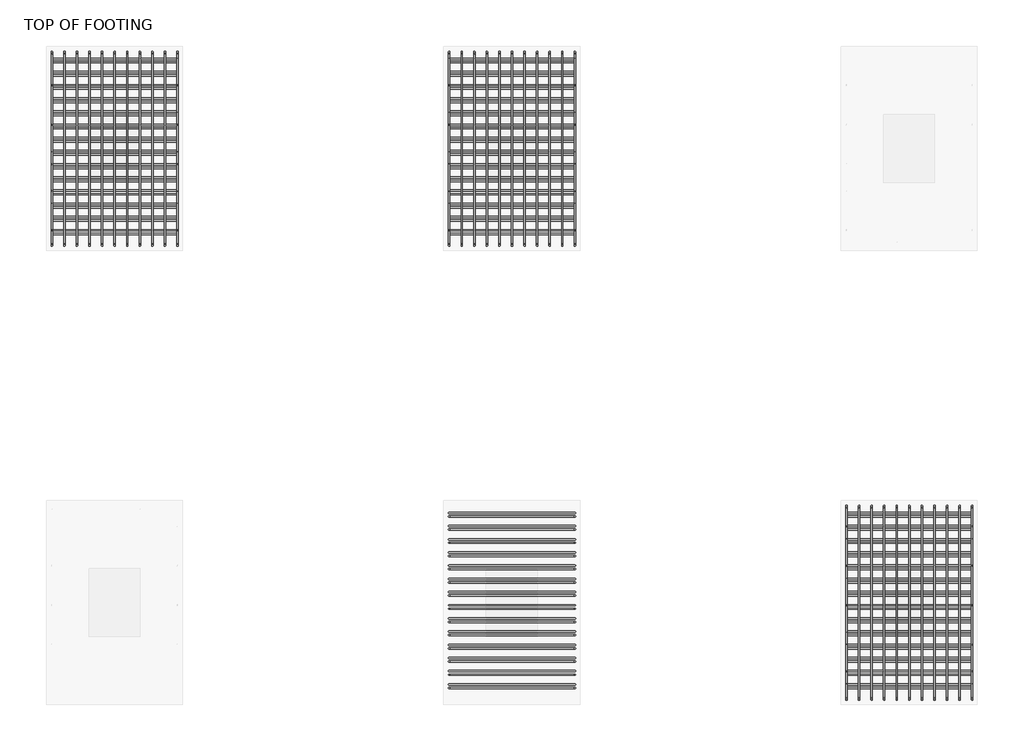
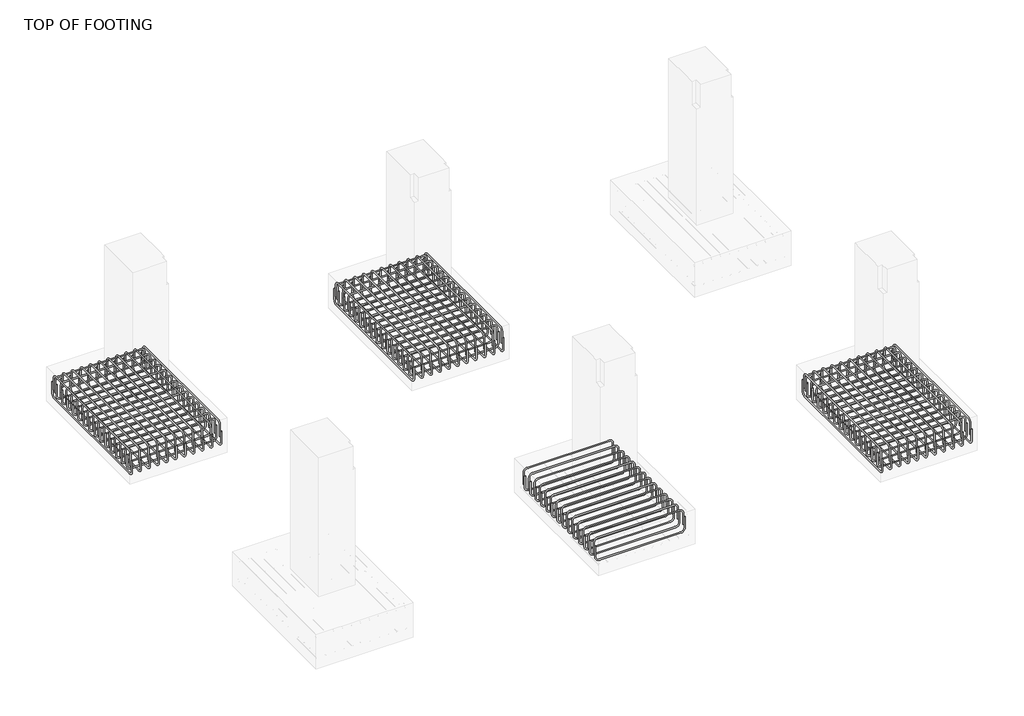
# One storey, part 6 of 11: 14 reinforcing bars.
"""IFC4 building model written with IfcOpenShell, lengths in millimetres."""

from ifc_helpers import new_model, si_unit, point, frame, origin, place, context, project, spatial, polyline, circle_curve, trimmed, segment, composite_curve, source, transform, mapped, element, save
from ifc_brep_helpers import swept_disk

model = new_model("IFC4")

# Units and contexts
model_context = context("Model", 3, world=origin())
ifc_project = project(units=[si_unit("LENGTHUNIT", "METRE", prefix="MILLI")], contexts=[model_context])

# Site, building, storey
site = spatial("IfcSite", under=ifc_project)
building = spatial("IfcBuilding", under=site)
storey = spatial("IfcBuildingStorey", under=building, Name="TOP OF FOOTING", Elevation=-1828.8)

# Reinforcing bars
placement = place(None, origin())
reinforcing_bar_shape = source(origin(), model_context, "Body", "SolidModel", [
    swept_disk(composite_curve([segment(polyline([(-8816.2384094, 18549.4712443, -2012.1658531), (-8816.2384094, 18549.4712443, -2159.4658531)]), True, "CONTINUOUS"), segment(trimmed(circle_curve(frame((-8816.2384094, 18595.8212443, -2159.4658531), z_axis=(1.0, 0.0, 0.0), x_axis=(0.0, -46.35000000000218, 0.0)), 46.35), [point((-8816.2384094, 18549.4712443, -2159.4658531))], [point((-8816.2384094, 18595.8212443, -2205.8158531))], True, "CARTESIAN"), True, "CONTINUOUS"), segment(polyline([(-8816.2384094, 18595.8212443, -2205.8158531), (-8816.2384094, 20210.4212443, -2205.8158531)]), True, "CONTINUOUS"), segment(trimmed(circle_curve(frame((-8816.2384094, 20210.4212443, -2159.4658531), z_axis=(1.0, 0.0, 0.0), x_axis=(0.0, 0.0, -46.34999999999991)), 46.35), [point((-8816.2384094, 20210.4212443, -2205.8158531))], [point((-8816.2384094, 20256.7712443, -2159.4658531))], True, "CARTESIAN"), True, "CONTINUOUS"), segment(polyline([(-8816.2384094, 20256.7712443, -2159.4658531), (-8816.2384094, 20256.7712443, -2012.1658531)]), True, "CONTINUOUS")], self_intersect=False), 6.35),
])
element("IfcReinforcingBar", 1, at=placement, inside=storey, context=model_context, shape_type="MappedRepresentation", body=[
    mapped(reinforcing_bar_shape, transform((0.0, 0.0, 0.0), x_axis=(1.0, 0.0, 0.0), y_axis=(0.0, 1.0, 0.0), z_axis=(0.0, 0.0, 1.0))),
    mapped(reinforcing_bar_shape, transform((-110.73, 0.0, 0.0), x_axis=(1.0, 0.0, 0.0), y_axis=(0.0, 1.0, 0.0), z_axis=(0.0, 0.0, 1.0))),
    mapped(reinforcing_bar_shape, transform((-221.46, 0.0, 0.0), x_axis=(1.0, 0.0, 0.0), y_axis=(0.0, 1.0, 0.0), z_axis=(0.0, 0.0, 1.0))),
    mapped(reinforcing_bar_shape, transform((-332.19, 0.0, 0.0), x_axis=(1.0, 0.0, 0.0), y_axis=(0.0, 1.0, 0.0), z_axis=(0.0, 0.0, 1.0))),
    mapped(reinforcing_bar_shape, transform((-442.92, 0.0, 0.0), x_axis=(1.0, 0.0, 0.0), y_axis=(0.0, 1.0, 0.0), z_axis=(0.0, 0.0, 1.0))),
    mapped(reinforcing_bar_shape, transform((-553.65, 0.0, 0.0), x_axis=(1.0, 0.0, 0.0), y_axis=(0.0, 1.0, 0.0), z_axis=(0.0, 0.0, 1.0))),
    mapped(reinforcing_bar_shape, transform((-664.38, 0.0, 0.0), x_axis=(1.0, 0.0, 0.0), y_axis=(0.0, 1.0, 0.0), z_axis=(0.0, 0.0, 1.0))),
    mapped(reinforcing_bar_shape, transform((-775.11, 0.0, 0.0), x_axis=(1.0, 0.0, 0.0), y_axis=(0.0, 1.0, 0.0), z_axis=(0.0, 0.0, 1.0))),
    mapped(reinforcing_bar_shape, transform((-885.84, 0.0, 0.0), x_axis=(1.0, 0.0, 0.0), y_axis=(0.0, 1.0, 0.0), z_axis=(0.0, 0.0, 1.0))),
    mapped(reinforcing_bar_shape, transform((-996.57, 0.0, 0.0), x_axis=(1.0, 0.0, 0.0), y_axis=(0.0, 1.0, 0.0), z_axis=(0.0, 0.0, 1.0))),
    mapped(reinforcing_bar_shape, transform((-1107.3, 0.0, 0.0), x_axis=(1.0, 0.0, 0.0), y_axis=(0.0, 1.0, 0.0), z_axis=(0.0, 0.0, 1.0))),
])
reinforcing_bar_2_shape = source(origin(), model_context, "Body", "SolidModel", [
    swept_disk(composite_curve([segment(polyline([(-9923.5384094, 18577.6603603, -2096.8914539), (-9923.5384094, 18577.6603603, -1949.5914539)]), True, "CONTINUOUS"), segment(trimmed(circle_curve(frame((-9923.5384094, 18624.0103603, -1949.5914539), z_axis=(-1.0, 0.0, 0.0), x_axis=(0.0, -46.349999999998545, 0.0)), 46.35), [point((-9923.5384094, 18577.6603603, -1949.5914539))], [point((-9923.5384094, 18624.0103603, -1903.2414539))], True, "CARTESIAN"), True, "CONTINUOUS"), segment(polyline([(-9923.5384094, 18624.0103603, -1903.2414539), (-9923.5384094, 20181.3238837, -1903.2414539)]), True, "CONTINUOUS"), segment(trimmed(circle_curve(frame((-9923.5384094, 20181.3238837, -1949.5914539), z_axis=(-1.0, 0.0, 0.0), x_axis=(0.0, 0.0, 46.350000000000136)), 46.35), [point((-9923.5384094, 20181.3238837, -1903.2414539))], [point((-9923.5384094, 20227.6738837, -1949.5914539))], True, "CARTESIAN"), True, "CONTINUOUS"), segment(polyline([(-9923.5384094, 20227.6738837, -1949.5914539), (-9923.5384094, 20227.6738837, -2096.8914539)]), True, "CONTINUOUS")], self_intersect=False), 6.35),
])
element("IfcReinforcingBar", 2, at=placement, inside=storey, context=model_context, shape_type="MappedRepresentation", body=[
    mapped(reinforcing_bar_2_shape, transform((0.0, 0.0, 0.0), x_axis=(1.0, 0.0, 0.0), y_axis=(0.0, 1.0, 0.0), z_axis=(0.0, 0.0, 1.0))),
    mapped(reinforcing_bar_2_shape, transform((110.73, 0.0, 0.0), x_axis=(1.0, 0.0, 0.0), y_axis=(0.0, 1.0, 0.0), z_axis=(0.0, 0.0, 1.0))),
    mapped(reinforcing_bar_2_shape, transform((221.46, 0.0, 0.0), x_axis=(1.0, 0.0, 0.0), y_axis=(0.0, 1.0, 0.0), z_axis=(0.0, 0.0, 1.0))),
    mapped(reinforcing_bar_2_shape, transform((332.19, 0.0, 0.0), x_axis=(1.0, 0.0, 0.0), y_axis=(0.0, 1.0, 0.0), z_axis=(0.0, 0.0, 1.0))),
    mapped(reinforcing_bar_2_shape, transform((442.92, 0.0, 0.0), x_axis=(1.0, 0.0, 0.0), y_axis=(0.0, 1.0, 0.0), z_axis=(0.0, 0.0, 1.0))),
    mapped(reinforcing_bar_2_shape, transform((553.65, 0.0, 0.0), x_axis=(1.0, 0.0, 0.0), y_axis=(0.0, 1.0, 0.0), z_axis=(0.0, 0.0, 1.0))),
    mapped(reinforcing_bar_2_shape, transform((664.38, 0.0, 0.0), x_axis=(1.0, 0.0, 0.0), y_axis=(0.0, 1.0, 0.0), z_axis=(0.0, 0.0, 1.0))),
    mapped(reinforcing_bar_2_shape, transform((775.11, 0.0, 0.0), x_axis=(1.0, 0.0, 0.0), y_axis=(0.0, 1.0, 0.0), z_axis=(0.0, 0.0, 1.0))),
    mapped(reinforcing_bar_2_shape, transform((885.84, 0.0, 0.0), x_axis=(1.0, 0.0, 0.0), y_axis=(0.0, 1.0, 0.0), z_axis=(0.0, 0.0, 1.0))),
    mapped(reinforcing_bar_2_shape, transform((996.57, 0.0, 0.0), x_axis=(1.0, 0.0, 0.0), y_axis=(0.0, 1.0, 0.0), z_axis=(0.0, 0.0, 1.0))),
    mapped(reinforcing_bar_2_shape, transform((1107.3, 0.0, 0.0), x_axis=(1.0, 0.0, 0.0), y_axis=(0.0, 1.0, 0.0), z_axis=(0.0, 0.0, 1.0))),
])
reinforcing_bar_3_shape = source(origin(), model_context, "Body", "SolidModel", [
    swept_disk(composite_curve([segment(polyline([(-9923.5384094, 18653.1930221, -1996.7664426), (-9923.5384094, 18653.1930221, -2144.0664426)]), True, "CONTINUOUS"), segment(trimmed(circle_curve(frame((-9877.1884094, 18653.1930221, -2144.0664426), z_axis=(0.0, -1.0, 0.0), x_axis=(-46.350000000000364, 0.0, 0.0)), 46.35), [point((-9923.5384094, 18653.1930221, -2144.0664426))], [point((-9877.1884094, 18653.1930221, -2190.4164426))], True, "CARTESIAN"), True, "CONTINUOUS"), segment(polyline([(-9877.1884094, 18653.1930221, -2190.4164426), (-8862.5884094, 18653.1930221, -2190.4164426)]), True, "CONTINUOUS"), segment(trimmed(circle_curve(frame((-8862.5884094, 18653.1930221, -2144.0664426), z_axis=(0.0, -1.0, 0.0), x_axis=(0.0, 0.0, -46.350000000000364)), 46.35), [point((-8862.5884094, 18653.1930221, -2190.4164426))], [point((-8816.2384094, 18653.1930221, -2144.0664426))], True, "CARTESIAN"), True, "CONTINUOUS"), segment(polyline([(-8816.2384094, 18653.1930221, -2144.0664426), (-8816.2384094, 18653.1930221, -1996.7664426)]), True, "CONTINUOUS")], self_intersect=False), 6.35),
])
element("IfcReinforcingBar", 3, at=placement, inside=storey, context=model_context, shape_type="MappedRepresentation", body=[
    mapped(reinforcing_bar_3_shape, transform((0.0, 0.0, 0.0), x_axis=(1.0, 0.0, 0.0), y_axis=(0.0, 1.0, 0.0), z_axis=(0.0, 0.0, 1.0))),
    mapped(reinforcing_bar_3_shape, transform((0.0, 116.2744005, 0.0), x_axis=(1.0, 0.0, 0.0), y_axis=(0.0, 1.0, 0.0), z_axis=(0.0, 0.0, 1.0))),
    mapped(reinforcing_bar_3_shape, transform((0.0, 232.5488009, 0.0), x_axis=(1.0, 0.0, 0.0), y_axis=(0.0, 1.0, 0.0), z_axis=(0.0, 0.0, 1.0))),
    mapped(reinforcing_bar_3_shape, transform((0.0, 348.8232014, 0.0), x_axis=(1.0, 0.0, 0.0), y_axis=(0.0, 1.0, 0.0), z_axis=(0.0, 0.0, 1.0))),
    mapped(reinforcing_bar_3_shape, transform((0.0, 465.0976018, 0.0), x_axis=(1.0, 0.0, 0.0), y_axis=(0.0, 1.0, 0.0), z_axis=(0.0, 0.0, 1.0))),
    mapped(reinforcing_bar_3_shape, transform((0.0, 581.3720023, 0.0), x_axis=(1.0, 0.0, 0.0), y_axis=(0.0, 1.0, 0.0), z_axis=(0.0, 0.0, 1.0))),
    mapped(reinforcing_bar_3_shape, transform((0.0, 697.6464027, 0.0), x_axis=(1.0, 0.0, 0.0), y_axis=(0.0, 1.0, 0.0), z_axis=(0.0, 0.0, 1.0))),
    mapped(reinforcing_bar_3_shape, transform((0.0, 813.9208032, 0.0), x_axis=(1.0, 0.0, 0.0), y_axis=(0.0, 1.0, 0.0), z_axis=(0.0, 0.0, 1.0))),
    mapped(reinforcing_bar_3_shape, transform((0.0, 930.1952036, 0.0), x_axis=(1.0, 0.0, 0.0), y_axis=(0.0, 1.0, 0.0), z_axis=(0.0, 0.0, 1.0))),
    mapped(reinforcing_bar_3_shape, transform((0.0, 1046.4696041, 0.0), x_axis=(1.0, 0.0, 0.0), y_axis=(0.0, 1.0, 0.0), z_axis=(0.0, 0.0, 1.0))),
    mapped(reinforcing_bar_3_shape, transform((0.0, 1162.7440045, 0.0), x_axis=(1.0, 0.0, 0.0), y_axis=(0.0, 1.0, 0.0), z_axis=(0.0, 0.0, 1.0))),
    mapped(reinforcing_bar_3_shape, transform((0.0, 1279.018405, 0.0), x_axis=(1.0, 0.0, 0.0), y_axis=(0.0, 1.0, 0.0), z_axis=(0.0, 0.0, 1.0))),
    mapped(reinforcing_bar_3_shape, transform((0.0, 1395.2928054, 0.0), x_axis=(1.0, 0.0, 0.0), y_axis=(0.0, 1.0, 0.0), z_axis=(0.0, 0.0, 1.0))),
    mapped(reinforcing_bar_3_shape, transform((0.0, 1511.5672059, 0.0), x_axis=(1.0, 0.0, 0.0), y_axis=(0.0, 1.0, 0.0), z_axis=(0.0, 0.0, 1.0))),
])
reinforcing_bar_4_shape = source(origin(), model_context, "Body", "SolidModel", [
    swept_disk(composite_curve([segment(polyline([(-9923.5384094, 20194.4257435, -2114.1958609), (-9923.5384094, 20194.4257435, -1966.8958609)]), True, "CONTINUOUS"), segment(trimmed(circle_curve(frame((-9877.1884094, 20194.4257435, -1966.8958609), z_axis=(0.0, 1.0, 0.0), x_axis=(-46.350000000000364, 0.0, 0.0)), 46.35), [point((-9923.5384094, 20194.4257435, -1966.8958609))], [point((-9877.1884094, 20194.4257435, -1920.5458609))], True, "CARTESIAN"), True, "CONTINUOUS"), segment(polyline([(-9877.1884094, 20194.4257435, -1920.5458609), (-8862.5884094, 20194.4257435, -1920.5458609)]), True, "CONTINUOUS"), segment(trimmed(circle_curve(frame((-8862.5884094, 20194.4257435, -1966.8958609), z_axis=(0.0, 1.0, 0.0), x_axis=(0.0, 0.0, 46.34999999999991)), 46.35), [point((-8862.5884094, 20194.4257435, -1920.5458609))], [point((-8816.2384094, 20194.4257435, -1966.8958609))], True, "CARTESIAN"), True, "CONTINUOUS"), segment(polyline([(-8816.2384094, 20194.4257435, -1966.8958609), (-8816.2384094, 20194.4257435, -2114.1958609)]), True, "CONTINUOUS")], self_intersect=False), 6.35),
])
element("IfcReinforcingBar", 4, at=placement, inside=storey, context=model_context, shape_type="MappedRepresentation", body=[
    mapped(reinforcing_bar_4_shape, transform((0.0, 0.0, 0.0), x_axis=(1.0, 0.0, 0.0), y_axis=(0.0, 1.0, 0.0), z_axis=(0.0, 0.0, 1.0))),
    mapped(reinforcing_bar_4_shape, transform((0.0, -116.1057918, 0.0), x_axis=(1.0, 0.0, 0.0), y_axis=(0.0, 1.0, 0.0), z_axis=(0.0, 0.0, 1.0))),
    mapped(reinforcing_bar_4_shape, transform((0.0, -232.2115836, 0.0), x_axis=(1.0, 0.0, 0.0), y_axis=(0.0, 1.0, 0.0), z_axis=(0.0, 0.0, 1.0))),
    mapped(reinforcing_bar_4_shape, transform((0.0, -348.3173754, 0.0), x_axis=(1.0, 0.0, 0.0), y_axis=(0.0, 1.0, 0.0), z_axis=(0.0, 0.0, 1.0))),
    mapped(reinforcing_bar_4_shape, transform((0.0, -464.4231672, 0.0), x_axis=(1.0, 0.0, 0.0), y_axis=(0.0, 1.0, 0.0), z_axis=(0.0, 0.0, 1.0))),
    mapped(reinforcing_bar_4_shape, transform((0.0, -580.528959, 0.0), x_axis=(1.0, 0.0, 0.0), y_axis=(0.0, 1.0, 0.0), z_axis=(0.0, 0.0, 1.0))),
    mapped(reinforcing_bar_4_shape, transform((0.0, -696.6347508, 0.0), x_axis=(1.0, 0.0, 0.0), y_axis=(0.0, 1.0, 0.0), z_axis=(0.0, 0.0, 1.0))),
    mapped(reinforcing_bar_4_shape, transform((0.0, -812.7405426, 0.0), x_axis=(1.0, 0.0, 0.0), y_axis=(0.0, 1.0, 0.0), z_axis=(0.0, 0.0, 1.0))),
    mapped(reinforcing_bar_4_shape, transform((0.0, -928.8463344, 0.0), x_axis=(1.0, 0.0, 0.0), y_axis=(0.0, 1.0, 0.0), z_axis=(0.0, 0.0, 1.0))),
    mapped(reinforcing_bar_4_shape, transform((0.0, -1044.9521262, 0.0), x_axis=(1.0, 0.0, 0.0), y_axis=(0.0, 1.0, 0.0), z_axis=(0.0, 0.0, 1.0))),
    mapped(reinforcing_bar_4_shape, transform((0.0, -1161.057918, 0.0), x_axis=(1.0, 0.0, 0.0), y_axis=(0.0, 1.0, 0.0), z_axis=(0.0, 0.0, 1.0))),
    mapped(reinforcing_bar_4_shape, transform((0.0, -1277.1637098, 0.0), x_axis=(1.0, 0.0, 0.0), y_axis=(0.0, 1.0, 0.0), z_axis=(0.0, 0.0, 1.0))),
    mapped(reinforcing_bar_4_shape, transform((0.0, -1393.2695016, 0.0), x_axis=(1.0, 0.0, 0.0), y_axis=(0.0, 1.0, 0.0), z_axis=(0.0, 0.0, 1.0))),
    mapped(reinforcing_bar_4_shape, transform((0.0, -1509.3752934, 0.0), x_axis=(1.0, 0.0, 0.0), y_axis=(0.0, 1.0, 0.0), z_axis=(0.0, 0.0, 1.0))),
])
reinforcing_bar_5_shape = source(origin(), model_context, "Body", "SolidModel", [
    swept_disk(composite_curve([segment(polyline([(-5316.2384094, 18549.4712443, -2012.1658531), (-5316.2384094, 18549.4712443, -2159.4658531)]), True, "CONTINUOUS"), segment(trimmed(circle_curve(frame((-5316.2384094, 18595.8212443, -2159.4658531), z_axis=(1.0, 0.0, 0.0), x_axis=(0.0, -46.35000000000218, 0.0)), 46.35), [point((-5316.2384094, 18549.4712443, -2159.4658531))], [point((-5316.2384094, 18595.8212443, -2205.8158531))], True, "CARTESIAN"), True, "CONTINUOUS"), segment(polyline([(-5316.2384094, 18595.8212443, -2205.8158531), (-5316.2384094, 20210.4212443, -2205.8158531)]), True, "CONTINUOUS"), segment(trimmed(circle_curve(frame((-5316.2384094, 20210.4212443, -2159.4658531), z_axis=(1.0, 0.0, 0.0), x_axis=(0.0, 0.0, -46.34999999999991)), 46.35), [point((-5316.2384094, 20210.4212443, -2205.8158531))], [point((-5316.2384094, 20256.7712443, -2159.4658531))], True, "CARTESIAN"), True, "CONTINUOUS"), segment(polyline([(-5316.2384094, 20256.7712443, -2159.4658531), (-5316.2384094, 20256.7712443, -2012.1658531)]), True, "CONTINUOUS")], self_intersect=False), 6.35),
])
element("IfcReinforcingBar", 5, at=placement, inside=storey, context=model_context, shape_type="MappedRepresentation", body=[
    mapped(reinforcing_bar_5_shape, transform((0.0, 0.0, 0.0), x_axis=(1.0, 0.0, 0.0), y_axis=(0.0, 1.0, 0.0), z_axis=(0.0, 0.0, 1.0))),
    mapped(reinforcing_bar_5_shape, transform((-110.73, 0.0, 0.0), x_axis=(1.0, 0.0, 0.0), y_axis=(0.0, 1.0, 0.0), z_axis=(0.0, 0.0, 1.0))),
    mapped(reinforcing_bar_5_shape, transform((-221.46, 0.0, 0.0), x_axis=(1.0, 0.0, 0.0), y_axis=(0.0, 1.0, 0.0), z_axis=(0.0, 0.0, 1.0))),
    mapped(reinforcing_bar_5_shape, transform((-332.19, 0.0, 0.0), x_axis=(1.0, 0.0, 0.0), y_axis=(0.0, 1.0, 0.0), z_axis=(0.0, 0.0, 1.0))),
    mapped(reinforcing_bar_5_shape, transform((-442.92, 0.0, 0.0), x_axis=(1.0, 0.0, 0.0), y_axis=(0.0, 1.0, 0.0), z_axis=(0.0, 0.0, 1.0))),
    mapped(reinforcing_bar_5_shape, transform((-553.65, 0.0, 0.0), x_axis=(1.0, 0.0, 0.0), y_axis=(0.0, 1.0, 0.0), z_axis=(0.0, 0.0, 1.0))),
    mapped(reinforcing_bar_5_shape, transform((-664.38, 0.0, 0.0), x_axis=(1.0, 0.0, 0.0), y_axis=(0.0, 1.0, 0.0), z_axis=(0.0, 0.0, 1.0))),
    mapped(reinforcing_bar_5_shape, transform((-775.11, 0.0, 0.0), x_axis=(1.0, 0.0, 0.0), y_axis=(0.0, 1.0, 0.0), z_axis=(0.0, 0.0, 1.0))),
    mapped(reinforcing_bar_5_shape, transform((-885.84, 0.0, 0.0), x_axis=(1.0, 0.0, 0.0), y_axis=(0.0, 1.0, 0.0), z_axis=(0.0, 0.0, 1.0))),
    mapped(reinforcing_bar_5_shape, transform((-996.57, 0.0, 0.0), x_axis=(1.0, 0.0, 0.0), y_axis=(0.0, 1.0, 0.0), z_axis=(0.0, 0.0, 1.0))),
    mapped(reinforcing_bar_5_shape, transform((-1107.3, 0.0, 0.0), x_axis=(1.0, 0.0, 0.0), y_axis=(0.0, 1.0, 0.0), z_axis=(0.0, 0.0, 1.0))),
])
reinforcing_bar_6_shape = source(origin(), model_context, "Body", "SolidModel", [
    swept_disk(composite_curve([segment(polyline([(-6423.5384094, 18577.6603603, -2096.8914539), (-6423.5384094, 18577.6603603, -1949.5914539)]), True, "CONTINUOUS"), segment(trimmed(circle_curve(frame((-6423.5384094, 18624.0103603, -1949.5914539), z_axis=(-1.0, 0.0, 0.0), x_axis=(0.0, -46.349999999998545, 0.0)), 46.35), [point((-6423.5384094, 18577.6603603, -1949.5914539))], [point((-6423.5384094, 18624.0103603, -1903.2414539))], True, "CARTESIAN"), True, "CONTINUOUS"), segment(polyline([(-6423.5384094, 18624.0103603, -1903.2414539), (-6423.5384094, 20181.3238837, -1903.2414539)]), True, "CONTINUOUS"), segment(trimmed(circle_curve(frame((-6423.5384094, 20181.3238837, -1949.5914539), z_axis=(-1.0, 0.0, 0.0), x_axis=(0.0, 0.0, 46.350000000000136)), 46.35), [point((-6423.5384094, 20181.3238837, -1903.2414539))], [point((-6423.5384094, 20227.6738837, -1949.5914539))], True, "CARTESIAN"), True, "CONTINUOUS"), segment(polyline([(-6423.5384094, 20227.6738837, -1949.5914539), (-6423.5384094, 20227.6738837, -2096.8914539)]), True, "CONTINUOUS")], self_intersect=False), 6.35),
])
element("IfcReinforcingBar", 6, at=placement, inside=storey, context=model_context, shape_type="MappedRepresentation", body=[
    mapped(reinforcing_bar_6_shape, transform((0.0, 0.0, 0.0), x_axis=(1.0, 0.0, 0.0), y_axis=(0.0, 1.0, 0.0), z_axis=(0.0, 0.0, 1.0))),
    mapped(reinforcing_bar_6_shape, transform((110.73, 0.0, 0.0), x_axis=(1.0, 0.0, 0.0), y_axis=(0.0, 1.0, 0.0), z_axis=(0.0, 0.0, 1.0))),
    mapped(reinforcing_bar_6_shape, transform((221.46, 0.0, 0.0), x_axis=(1.0, 0.0, 0.0), y_axis=(0.0, 1.0, 0.0), z_axis=(0.0, 0.0, 1.0))),
    mapped(reinforcing_bar_6_shape, transform((332.19, 0.0, 0.0), x_axis=(1.0, 0.0, 0.0), y_axis=(0.0, 1.0, 0.0), z_axis=(0.0, 0.0, 1.0))),
    mapped(reinforcing_bar_6_shape, transform((442.92, 0.0, 0.0), x_axis=(1.0, 0.0, 0.0), y_axis=(0.0, 1.0, 0.0), z_axis=(0.0, 0.0, 1.0))),
    mapped(reinforcing_bar_6_shape, transform((553.65, 0.0, 0.0), x_axis=(1.0, 0.0, 0.0), y_axis=(0.0, 1.0, 0.0), z_axis=(0.0, 0.0, 1.0))),
    mapped(reinforcing_bar_6_shape, transform((664.38, 0.0, 0.0), x_axis=(1.0, 0.0, 0.0), y_axis=(0.0, 1.0, 0.0), z_axis=(0.0, 0.0, 1.0))),
    mapped(reinforcing_bar_6_shape, transform((775.11, 0.0, 0.0), x_axis=(1.0, 0.0, 0.0), y_axis=(0.0, 1.0, 0.0), z_axis=(0.0, 0.0, 1.0))),
    mapped(reinforcing_bar_6_shape, transform((885.84, 0.0, 0.0), x_axis=(1.0, 0.0, 0.0), y_axis=(0.0, 1.0, 0.0), z_axis=(0.0, 0.0, 1.0))),
    mapped(reinforcing_bar_6_shape, transform((996.57, 0.0, 0.0), x_axis=(1.0, 0.0, 0.0), y_axis=(0.0, 1.0, 0.0), z_axis=(0.0, 0.0, 1.0))),
    mapped(reinforcing_bar_6_shape, transform((1107.3, 0.0, 0.0), x_axis=(1.0, 0.0, 0.0), y_axis=(0.0, 1.0, 0.0), z_axis=(0.0, 0.0, 1.0))),
])
reinforcing_bar_7_shape = source(origin(), model_context, "Body", "SolidModel", [
    swept_disk(composite_curve([segment(polyline([(-6423.5384094, 18653.1930221, -1996.7664426), (-6423.5384094, 18653.1930221, -2144.0664426)]), True, "CONTINUOUS"), segment(trimmed(circle_curve(frame((-6377.1884094, 18653.1930221, -2144.0664426), z_axis=(0.0, -1.0, 0.0), x_axis=(-46.350000000000364, 0.0, 0.0)), 46.35), [point((-6423.5384094, 18653.1930221, -2144.0664426))], [point((-6377.1884094, 18653.1930221, -2190.4164426))], True, "CARTESIAN"), True, "CONTINUOUS"), segment(polyline([(-6377.1884094, 18653.1930221, -2190.4164426), (-5362.5884094, 18653.1930221, -2190.4164426)]), True, "CONTINUOUS"), segment(trimmed(circle_curve(frame((-5362.5884094, 18653.1930221, -2144.0664426), z_axis=(0.0, -1.0, 0.0), x_axis=(0.0, 0.0, -46.350000000000364)), 46.35), [point((-5362.5884094, 18653.1930221, -2190.4164426))], [point((-5316.2384094, 18653.1930221, -2144.0664426))], True, "CARTESIAN"), True, "CONTINUOUS"), segment(polyline([(-5316.2384094, 18653.1930221, -2144.0664426), (-5316.2384094, 18653.1930221, -1996.7664426)]), True, "CONTINUOUS")], self_intersect=False), 6.35),
])
element("IfcReinforcingBar", 7, at=placement, inside=storey, context=model_context, shape_type="MappedRepresentation", body=[
    mapped(reinforcing_bar_7_shape, transform((0.0, 0.0, 0.0), x_axis=(1.0, 0.0, 0.0), y_axis=(0.0, 1.0, 0.0), z_axis=(0.0, 0.0, 1.0))),
    mapped(reinforcing_bar_7_shape, transform((0.0, 116.2744005, 0.0), x_axis=(1.0, 0.0, 0.0), y_axis=(0.0, 1.0, 0.0), z_axis=(0.0, 0.0, 1.0))),
    mapped(reinforcing_bar_7_shape, transform((0.0, 232.5488009, 0.0), x_axis=(1.0, 0.0, 0.0), y_axis=(0.0, 1.0, 0.0), z_axis=(0.0, 0.0, 1.0))),
    mapped(reinforcing_bar_7_shape, transform((0.0, 348.8232014, 0.0), x_axis=(1.0, 0.0, 0.0), y_axis=(0.0, 1.0, 0.0), z_axis=(0.0, 0.0, 1.0))),
    mapped(reinforcing_bar_7_shape, transform((0.0, 465.0976018, 0.0), x_axis=(1.0, 0.0, 0.0), y_axis=(0.0, 1.0, 0.0), z_axis=(0.0, 0.0, 1.0))),
    mapped(reinforcing_bar_7_shape, transform((0.0, 581.3720023, 0.0), x_axis=(1.0, 0.0, 0.0), y_axis=(0.0, 1.0, 0.0), z_axis=(0.0, 0.0, 1.0))),
    mapped(reinforcing_bar_7_shape, transform((0.0, 697.6464027, 0.0), x_axis=(1.0, 0.0, 0.0), y_axis=(0.0, 1.0, 0.0), z_axis=(0.0, 0.0, 1.0))),
    mapped(reinforcing_bar_7_shape, transform((0.0, 813.9208032, 0.0), x_axis=(1.0, 0.0, 0.0), y_axis=(0.0, 1.0, 0.0), z_axis=(0.0, 0.0, 1.0))),
    mapped(reinforcing_bar_7_shape, transform((0.0, 930.1952036, 0.0), x_axis=(1.0, 0.0, 0.0), y_axis=(0.0, 1.0, 0.0), z_axis=(0.0, 0.0, 1.0))),
    mapped(reinforcing_bar_7_shape, transform((0.0, 1046.4696041, 0.0), x_axis=(1.0, 0.0, 0.0), y_axis=(0.0, 1.0, 0.0), z_axis=(0.0, 0.0, 1.0))),
    mapped(reinforcing_bar_7_shape, transform((0.0, 1162.7440045, 0.0), x_axis=(1.0, 0.0, 0.0), y_axis=(0.0, 1.0, 0.0), z_axis=(0.0, 0.0, 1.0))),
    mapped(reinforcing_bar_7_shape, transform((0.0, 1279.018405, 0.0), x_axis=(1.0, 0.0, 0.0), y_axis=(0.0, 1.0, 0.0), z_axis=(0.0, 0.0, 1.0))),
    mapped(reinforcing_bar_7_shape, transform((0.0, 1395.2928054, 0.0), x_axis=(1.0, 0.0, 0.0), y_axis=(0.0, 1.0, 0.0), z_axis=(0.0, 0.0, 1.0))),
    mapped(reinforcing_bar_7_shape, transform((0.0, 1511.5672059, 0.0), x_axis=(1.0, 0.0, 0.0), y_axis=(0.0, 1.0, 0.0), z_axis=(0.0, 0.0, 1.0))),
])
reinforcing_bar_8_shape = source(origin(), model_context, "Body", "SolidModel", [
    swept_disk(composite_curve([segment(polyline([(-6423.5384094, 20194.4257435, -2114.1958609), (-6423.5384094, 20194.4257435, -1966.8958609)]), True, "CONTINUOUS"), segment(trimmed(circle_curve(frame((-6377.1884094, 20194.4257435, -1966.8958609), z_axis=(0.0, 1.0, 0.0), x_axis=(-46.350000000000364, 0.0, 0.0)), 46.35), [point((-6423.5384094, 20194.4257435, -1966.8958609))], [point((-6377.1884094, 20194.4257435, -1920.5458609))], True, "CARTESIAN"), True, "CONTINUOUS"), segment(polyline([(-6377.1884094, 20194.4257435, -1920.5458609), (-5362.5884094, 20194.4257435, -1920.5458609)]), True, "CONTINUOUS"), segment(trimmed(circle_curve(frame((-5362.5884094, 20194.4257435, -1966.8958609), z_axis=(0.0, 1.0, 0.0), x_axis=(0.0, 0.0, 46.34999999999991)), 46.35), [point((-5362.5884094, 20194.4257435, -1920.5458609))], [point((-5316.2384094, 20194.4257435, -1966.8958609))], True, "CARTESIAN"), True, "CONTINUOUS"), segment(polyline([(-5316.2384094, 20194.4257435, -1966.8958609), (-5316.2384094, 20194.4257435, -2114.1958609)]), True, "CONTINUOUS")], self_intersect=False), 6.35),
])
element("IfcReinforcingBar", 8, at=placement, inside=storey, context=model_context, shape_type="MappedRepresentation", body=[
    mapped(reinforcing_bar_8_shape, transform((0.0, 0.0, 0.0), x_axis=(1.0, 0.0, 0.0), y_axis=(0.0, 1.0, 0.0), z_axis=(0.0, 0.0, 1.0))),
    mapped(reinforcing_bar_8_shape, transform((0.0, -116.1057918, 0.0), x_axis=(1.0, 0.0, 0.0), y_axis=(0.0, 1.0, 0.0), z_axis=(0.0, 0.0, 1.0))),
    mapped(reinforcing_bar_8_shape, transform((0.0, -232.2115836, 0.0), x_axis=(1.0, 0.0, 0.0), y_axis=(0.0, 1.0, 0.0), z_axis=(0.0, 0.0, 1.0))),
    mapped(reinforcing_bar_8_shape, transform((0.0, -348.3173754, 0.0), x_axis=(1.0, 0.0, 0.0), y_axis=(0.0, 1.0, 0.0), z_axis=(0.0, 0.0, 1.0))),
    mapped(reinforcing_bar_8_shape, transform((0.0, -464.4231672, 0.0), x_axis=(1.0, 0.0, 0.0), y_axis=(0.0, 1.0, 0.0), z_axis=(0.0, 0.0, 1.0))),
    mapped(reinforcing_bar_8_shape, transform((0.0, -580.528959, 0.0), x_axis=(1.0, 0.0, 0.0), y_axis=(0.0, 1.0, 0.0), z_axis=(0.0, 0.0, 1.0))),
    mapped(reinforcing_bar_8_shape, transform((0.0, -696.6347508, 0.0), x_axis=(1.0, 0.0, 0.0), y_axis=(0.0, 1.0, 0.0), z_axis=(0.0, 0.0, 1.0))),
    mapped(reinforcing_bar_8_shape, transform((0.0, -812.7405426, 0.0), x_axis=(1.0, 0.0, 0.0), y_axis=(0.0, 1.0, 0.0), z_axis=(0.0, 0.0, 1.0))),
    mapped(reinforcing_bar_8_shape, transform((0.0, -928.8463344, 0.0), x_axis=(1.0, 0.0, 0.0), y_axis=(0.0, 1.0, 0.0), z_axis=(0.0, 0.0, 1.0))),
    mapped(reinforcing_bar_8_shape, transform((0.0, -1044.9521262, 0.0), x_axis=(1.0, 0.0, 0.0), y_axis=(0.0, 1.0, 0.0), z_axis=(0.0, 0.0, 1.0))),
    mapped(reinforcing_bar_8_shape, transform((0.0, -1161.057918, 0.0), x_axis=(1.0, 0.0, 0.0), y_axis=(0.0, 1.0, 0.0), z_axis=(0.0, 0.0, 1.0))),
    mapped(reinforcing_bar_8_shape, transform((0.0, -1277.1637098, 0.0), x_axis=(1.0, 0.0, 0.0), y_axis=(0.0, 1.0, 0.0), z_axis=(0.0, 0.0, 1.0))),
    mapped(reinforcing_bar_8_shape, transform((0.0, -1393.2695016, 0.0), x_axis=(1.0, 0.0, 0.0), y_axis=(0.0, 1.0, 0.0), z_axis=(0.0, 0.0, 1.0))),
    mapped(reinforcing_bar_8_shape, transform((0.0, -1509.3752934, 0.0), x_axis=(1.0, 0.0, 0.0), y_axis=(0.0, 1.0, 0.0), z_axis=(0.0, 0.0, 1.0))),
])
reinforcing_bar_9_shape = source(origin(), model_context, "Body", "SolidModel", [
    swept_disk(composite_curve([segment(polyline([(-6423.5384094, 14653.1930221, -1996.7664426), (-6423.5384094, 14653.1930221, -2144.0664426)]), True, "CONTINUOUS"), segment(trimmed(circle_curve(frame((-6377.1884094, 14653.1930221, -2144.0664426), z_axis=(0.0, -1.0, 0.0), x_axis=(-46.350000000000364, 0.0, 0.0)), 46.35), [point((-6423.5384094, 14653.1930221, -2144.0664426))], [point((-6377.1884094, 14653.1930221, -2190.4164426))], True, "CARTESIAN"), True, "CONTINUOUS"), segment(polyline([(-6377.1884094, 14653.1930221, -2190.4164426), (-5362.5884094, 14653.1930221, -2190.4164426)]), True, "CONTINUOUS"), segment(trimmed(circle_curve(frame((-5362.5884094, 14653.1930221, -2144.0664426), z_axis=(0.0, -1.0, 0.0), x_axis=(0.0, 0.0, -46.350000000000364)), 46.35), [point((-5362.5884094, 14653.1930221, -2190.4164426))], [point((-5316.2384094, 14653.1930221, -2144.0664426))], True, "CARTESIAN"), True, "CONTINUOUS"), segment(polyline([(-5316.2384094, 14653.1930221, -2144.0664426), (-5316.2384094, 14653.1930221, -1996.7664426)]), True, "CONTINUOUS")], self_intersect=False), 6.35),
])
element("IfcReinforcingBar", 9, at=placement, inside=storey, context=model_context, shape_type="MappedRepresentation", body=[
    mapped(reinforcing_bar_9_shape, transform((0.0, 0.0, 0.0), x_axis=(1.0, 0.0, 0.0), y_axis=(0.0, 1.0, 0.0), z_axis=(0.0, 0.0, 1.0))),
    mapped(reinforcing_bar_9_shape, transform((0.0, 116.2744005, 0.0), x_axis=(1.0, 0.0, 0.0), y_axis=(0.0, 1.0, 0.0), z_axis=(0.0, 0.0, 1.0))),
    mapped(reinforcing_bar_9_shape, transform((0.0, 232.5488009, 0.0), x_axis=(1.0, 0.0, 0.0), y_axis=(0.0, 1.0, 0.0), z_axis=(0.0, 0.0, 1.0))),
    mapped(reinforcing_bar_9_shape, transform((0.0, 348.8232014, 0.0), x_axis=(1.0, 0.0, 0.0), y_axis=(0.0, 1.0, 0.0), z_axis=(0.0, 0.0, 1.0))),
    mapped(reinforcing_bar_9_shape, transform((0.0, 465.0976018, 0.0), x_axis=(1.0, 0.0, 0.0), y_axis=(0.0, 1.0, 0.0), z_axis=(0.0, 0.0, 1.0))),
    mapped(reinforcing_bar_9_shape, transform((0.0, 581.3720023, 0.0), x_axis=(1.0, 0.0, 0.0), y_axis=(0.0, 1.0, 0.0), z_axis=(0.0, 0.0, 1.0))),
    mapped(reinforcing_bar_9_shape, transform((0.0, 697.6464027, 0.0), x_axis=(1.0, 0.0, 0.0), y_axis=(0.0, 1.0, 0.0), z_axis=(0.0, 0.0, 1.0))),
    mapped(reinforcing_bar_9_shape, transform((0.0, 813.9208032, 0.0), x_axis=(1.0, 0.0, 0.0), y_axis=(0.0, 1.0, 0.0), z_axis=(0.0, 0.0, 1.0))),
    mapped(reinforcing_bar_9_shape, transform((0.0, 930.1952036, 0.0), x_axis=(1.0, 0.0, 0.0), y_axis=(0.0, 1.0, 0.0), z_axis=(0.0, 0.0, 1.0))),
    mapped(reinforcing_bar_9_shape, transform((0.0, 1046.4696041, 0.0), x_axis=(1.0, 0.0, 0.0), y_axis=(0.0, 1.0, 0.0), z_axis=(0.0, 0.0, 1.0))),
    mapped(reinforcing_bar_9_shape, transform((0.0, 1162.7440045, 0.0), x_axis=(1.0, 0.0, 0.0), y_axis=(0.0, 1.0, 0.0), z_axis=(0.0, 0.0, 1.0))),
    mapped(reinforcing_bar_9_shape, transform((0.0, 1279.018405, 0.0), x_axis=(1.0, 0.0, 0.0), y_axis=(0.0, 1.0, 0.0), z_axis=(0.0, 0.0, 1.0))),
    mapped(reinforcing_bar_9_shape, transform((0.0, 1395.2928054, 0.0), x_axis=(1.0, 0.0, 0.0), y_axis=(0.0, 1.0, 0.0), z_axis=(0.0, 0.0, 1.0))),
    mapped(reinforcing_bar_9_shape, transform((0.0, 1511.5672059, 0.0), x_axis=(1.0, 0.0, 0.0), y_axis=(0.0, 1.0, 0.0), z_axis=(0.0, 0.0, 1.0))),
])
reinforcing_bar_10_shape = source(origin(), model_context, "Body", "SolidModel", [
    swept_disk(composite_curve([segment(polyline([(-6423.5384094, 16194.4257435, -2114.1958609), (-6423.5384094, 16194.4257435, -1966.8958609)]), True, "CONTINUOUS"), segment(trimmed(circle_curve(frame((-6377.1884094, 16194.4257435, -1966.8958609), z_axis=(0.0, 1.0, 0.0), x_axis=(-46.350000000000364, 0.0, 0.0)), 46.35), [point((-6423.5384094, 16194.4257435, -1966.8958609))], [point((-6377.1884094, 16194.4257435, -1920.5458609))], True, "CARTESIAN"), True, "CONTINUOUS"), segment(polyline([(-6377.1884094, 16194.4257435, -1920.5458609), (-5362.5884094, 16194.4257435, -1920.5458609)]), True, "CONTINUOUS"), segment(trimmed(circle_curve(frame((-5362.5884094, 16194.4257435, -1966.8958609), z_axis=(0.0, 1.0, 0.0), x_axis=(0.0, 0.0, 46.34999999999991)), 46.35), [point((-5362.5884094, 16194.4257435, -1920.5458609))], [point((-5316.2384094, 16194.4257435, -1966.8958609))], True, "CARTESIAN"), True, "CONTINUOUS"), segment(polyline([(-5316.2384094, 16194.4257435, -1966.8958609), (-5316.2384094, 16194.4257435, -2114.1958609)]), True, "CONTINUOUS")], self_intersect=False), 6.35),
])
element("IfcReinforcingBar", 10, at=placement, inside=storey, context=model_context, shape_type="MappedRepresentation", body=[
    mapped(reinforcing_bar_10_shape, transform((0.0, 0.0, 0.0), x_axis=(1.0, 0.0, 0.0), y_axis=(0.0, 1.0, 0.0), z_axis=(0.0, 0.0, 1.0))),
    mapped(reinforcing_bar_10_shape, transform((0.0, -116.1057918, 0.0), x_axis=(1.0, 0.0, 0.0), y_axis=(0.0, 1.0, 0.0), z_axis=(0.0, 0.0, 1.0))),
    mapped(reinforcing_bar_10_shape, transform((0.0, -232.2115836, 0.0), x_axis=(1.0, 0.0, 0.0), y_axis=(0.0, 1.0, 0.0), z_axis=(0.0, 0.0, 1.0))),
    mapped(reinforcing_bar_10_shape, transform((0.0, -348.3173754, 0.0), x_axis=(1.0, 0.0, 0.0), y_axis=(0.0, 1.0, 0.0), z_axis=(0.0, 0.0, 1.0))),
    mapped(reinforcing_bar_10_shape, transform((0.0, -464.4231672, 0.0), x_axis=(1.0, 0.0, 0.0), y_axis=(0.0, 1.0, 0.0), z_axis=(0.0, 0.0, 1.0))),
    mapped(reinforcing_bar_10_shape, transform((0.0, -580.528959, 0.0), x_axis=(1.0, 0.0, 0.0), y_axis=(0.0, 1.0, 0.0), z_axis=(0.0, 0.0, 1.0))),
    mapped(reinforcing_bar_10_shape, transform((0.0, -696.6347508, 0.0), x_axis=(1.0, 0.0, 0.0), y_axis=(0.0, 1.0, 0.0), z_axis=(0.0, 0.0, 1.0))),
    mapped(reinforcing_bar_10_shape, transform((0.0, -812.7405426, 0.0), x_axis=(1.0, 0.0, 0.0), y_axis=(0.0, 1.0, 0.0), z_axis=(0.0, 0.0, 1.0))),
    mapped(reinforcing_bar_10_shape, transform((0.0, -928.8463344, 0.0), x_axis=(1.0, 0.0, 0.0), y_axis=(0.0, 1.0, 0.0), z_axis=(0.0, 0.0, 1.0))),
    mapped(reinforcing_bar_10_shape, transform((0.0, -1044.9521262, 0.0), x_axis=(1.0, 0.0, 0.0), y_axis=(0.0, 1.0, 0.0), z_axis=(0.0, 0.0, 1.0))),
    mapped(reinforcing_bar_10_shape, transform((0.0, -1161.057918, 0.0), x_axis=(1.0, 0.0, 0.0), y_axis=(0.0, 1.0, 0.0), z_axis=(0.0, 0.0, 1.0))),
    mapped(reinforcing_bar_10_shape, transform((0.0, -1277.1637098, 0.0), x_axis=(1.0, 0.0, 0.0), y_axis=(0.0, 1.0, 0.0), z_axis=(0.0, 0.0, 1.0))),
    mapped(reinforcing_bar_10_shape, transform((0.0, -1393.2695016, 0.0), x_axis=(1.0, 0.0, 0.0), y_axis=(0.0, 1.0, 0.0), z_axis=(0.0, 0.0, 1.0))),
    mapped(reinforcing_bar_10_shape, transform((0.0, -1509.3752934, 0.0), x_axis=(1.0, 0.0, 0.0), y_axis=(0.0, 1.0, 0.0), z_axis=(0.0, 0.0, 1.0))),
])
reinforcing_bar_11_shape = source(origin(), model_context, "Body", "SolidModel", [
    swept_disk(composite_curve([segment(polyline([(-1816.2384094, 14549.4712443, -2012.1658531), (-1816.2384094, 14549.4712443, -2159.4658531)]), True, "CONTINUOUS"), segment(trimmed(circle_curve(frame((-1816.2384094, 14595.8212443, -2159.4658531), z_axis=(1.0, 0.0, 0.0), x_axis=(0.0, -46.349999999998545, 0.0)), 46.35), [point((-1816.2384094, 14549.4712443, -2159.4658531))], [point((-1816.2384094, 14595.8212443, -2205.8158531))], True, "CARTESIAN"), True, "CONTINUOUS"), segment(polyline([(-1816.2384094, 14595.8212443, -2205.8158531), (-1816.2384094, 16210.4212443, -2205.8158531)]), True, "CONTINUOUS"), segment(trimmed(circle_curve(frame((-1816.2384094, 16210.4212443, -2159.4658531), z_axis=(1.0, 0.0, 0.0), x_axis=(0.0, 0.0, -46.34999999999991)), 46.35), [point((-1816.2384094, 16210.4212443, -2205.8158531))], [point((-1816.2384094, 16256.7712443, -2159.4658531))], True, "CARTESIAN"), True, "CONTINUOUS"), segment(polyline([(-1816.2384094, 16256.7712443, -2159.4658531), (-1816.2384094, 16256.7712443, -2012.1658531)]), True, "CONTINUOUS")], self_intersect=False), 6.35),
])
element("IfcReinforcingBar", 11, at=placement, inside=storey, context=model_context, shape_type="MappedRepresentation", body=[
    mapped(reinforcing_bar_11_shape, transform((0.0, 0.0, 0.0), x_axis=(1.0, 0.0, 0.0), y_axis=(0.0, 1.0, 0.0), z_axis=(0.0, 0.0, 1.0))),
    mapped(reinforcing_bar_11_shape, transform((-110.73, 0.0, 0.0), x_axis=(1.0, 0.0, 0.0), y_axis=(0.0, 1.0, 0.0), z_axis=(0.0, 0.0, 1.0))),
    mapped(reinforcing_bar_11_shape, transform((-221.46, 0.0, 0.0), x_axis=(1.0, 0.0, 0.0), y_axis=(0.0, 1.0, 0.0), z_axis=(0.0, 0.0, 1.0))),
    mapped(reinforcing_bar_11_shape, transform((-332.19, 0.0, 0.0), x_axis=(1.0, 0.0, 0.0), y_axis=(0.0, 1.0, 0.0), z_axis=(0.0, 0.0, 1.0))),
    mapped(reinforcing_bar_11_shape, transform((-442.92, 0.0, 0.0), x_axis=(1.0, 0.0, 0.0), y_axis=(0.0, 1.0, 0.0), z_axis=(0.0, 0.0, 1.0))),
    mapped(reinforcing_bar_11_shape, transform((-553.65, 0.0, 0.0), x_axis=(1.0, 0.0, 0.0), y_axis=(0.0, 1.0, 0.0), z_axis=(0.0, 0.0, 1.0))),
    mapped(reinforcing_bar_11_shape, transform((-664.38, 0.0, 0.0), x_axis=(1.0, 0.0, 0.0), y_axis=(0.0, 1.0, 0.0), z_axis=(0.0, 0.0, 1.0))),
    mapped(reinforcing_bar_11_shape, transform((-775.11, 0.0, 0.0), x_axis=(1.0, 0.0, 0.0), y_axis=(0.0, 1.0, 0.0), z_axis=(0.0, 0.0, 1.0))),
    mapped(reinforcing_bar_11_shape, transform((-885.84, 0.0, 0.0), x_axis=(1.0, 0.0, 0.0), y_axis=(0.0, 1.0, 0.0), z_axis=(0.0, 0.0, 1.0))),
    mapped(reinforcing_bar_11_shape, transform((-996.57, 0.0, 0.0), x_axis=(1.0, 0.0, 0.0), y_axis=(0.0, 1.0, 0.0), z_axis=(0.0, 0.0, 1.0))),
    mapped(reinforcing_bar_11_shape, transform((-1107.3, 0.0, 0.0), x_axis=(1.0, 0.0, 0.0), y_axis=(0.0, 1.0, 0.0), z_axis=(0.0, 0.0, 1.0))),
])
reinforcing_bar_12_shape = source(origin(), model_context, "Body", "SolidModel", [
    swept_disk(composite_curve([segment(polyline([(-2923.5384094, 14577.6603603, -2096.8914539), (-2923.5384094, 14577.6603603, -1949.5914539)]), True, "CONTINUOUS"), segment(trimmed(circle_curve(frame((-2923.5384094, 14624.0103603, -1949.5914539), z_axis=(-1.0, 0.0, 0.0), x_axis=(0.0, -46.350000000000364, 0.0)), 46.35), [point((-2923.5384094, 14577.6603603, -1949.5914539))], [point((-2923.5384094, 14624.0103603, -1903.2414539))], True, "CARTESIAN"), True, "CONTINUOUS"), segment(polyline([(-2923.5384094, 14624.0103603, -1903.2414539), (-2923.5384094, 16181.3238837, -1903.2414539)]), True, "CONTINUOUS"), segment(trimmed(circle_curve(frame((-2923.5384094, 16181.3238837, -1949.5914539), z_axis=(-1.0, 0.0, 0.0), x_axis=(0.0, 0.0, 46.350000000000136)), 46.35), [point((-2923.5384094, 16181.3238837, -1903.2414539))], [point((-2923.5384094, 16227.6738837, -1949.5914539))], True, "CARTESIAN"), True, "CONTINUOUS"), segment(polyline([(-2923.5384094, 16227.6738837, -1949.5914539), (-2923.5384094, 16227.6738837, -2096.8914539)]), True, "CONTINUOUS")], self_intersect=False), 6.35),
])
element("IfcReinforcingBar", 12, at=placement, inside=storey, context=model_context, shape_type="MappedRepresentation", body=[
    mapped(reinforcing_bar_12_shape, transform((0.0, 0.0, 0.0), x_axis=(1.0, 0.0, 0.0), y_axis=(0.0, 1.0, 0.0), z_axis=(0.0, 0.0, 1.0))),
    mapped(reinforcing_bar_12_shape, transform((110.73, 0.0, 0.0), x_axis=(1.0, 0.0, 0.0), y_axis=(0.0, 1.0, 0.0), z_axis=(0.0, 0.0, 1.0))),
    mapped(reinforcing_bar_12_shape, transform((221.46, 0.0, 0.0), x_axis=(1.0, 0.0, 0.0), y_axis=(0.0, 1.0, 0.0), z_axis=(0.0, 0.0, 1.0))),
    mapped(reinforcing_bar_12_shape, transform((332.19, 0.0, 0.0), x_axis=(1.0, 0.0, 0.0), y_axis=(0.0, 1.0, 0.0), z_axis=(0.0, 0.0, 1.0))),
    mapped(reinforcing_bar_12_shape, transform((442.92, 0.0, 0.0), x_axis=(1.0, 0.0, 0.0), y_axis=(0.0, 1.0, 0.0), z_axis=(0.0, 0.0, 1.0))),
    mapped(reinforcing_bar_12_shape, transform((553.65, 0.0, 0.0), x_axis=(1.0, 0.0, 0.0), y_axis=(0.0, 1.0, 0.0), z_axis=(0.0, 0.0, 1.0))),
    mapped(reinforcing_bar_12_shape, transform((664.38, 0.0, 0.0), x_axis=(1.0, 0.0, 0.0), y_axis=(0.0, 1.0, 0.0), z_axis=(0.0, 0.0, 1.0))),
    mapped(reinforcing_bar_12_shape, transform((775.11, 0.0, 0.0), x_axis=(1.0, 0.0, 0.0), y_axis=(0.0, 1.0, 0.0), z_axis=(0.0, 0.0, 1.0))),
    mapped(reinforcing_bar_12_shape, transform((885.84, 0.0, 0.0), x_axis=(1.0, 0.0, 0.0), y_axis=(0.0, 1.0, 0.0), z_axis=(0.0, 0.0, 1.0))),
    mapped(reinforcing_bar_12_shape, transform((996.57, 0.0, 0.0), x_axis=(1.0, 0.0, 0.0), y_axis=(0.0, 1.0, 0.0), z_axis=(0.0, 0.0, 1.0))),
    mapped(reinforcing_bar_12_shape, transform((1107.3, 0.0, 0.0), x_axis=(1.0, 0.0, 0.0), y_axis=(0.0, 1.0, 0.0), z_axis=(0.0, 0.0, 1.0))),
])
reinforcing_bar_13_shape = source(origin(), model_context, "Body", "SolidModel", [
    swept_disk(composite_curve([segment(polyline([(-2923.5384094, 14653.1930221, -1996.7664426), (-2923.5384094, 14653.1930221, -2144.0664426)]), True, "CONTINUOUS"), segment(trimmed(circle_curve(frame((-2877.1884094, 14653.1930221, -2144.0664426), z_axis=(0.0, -1.0, 0.0), x_axis=(-46.34999999999991, 0.0, 0.0)), 46.35), [point((-2923.5384094, 14653.1930221, -2144.0664426))], [point((-2877.1884094, 14653.1930221, -2190.4164426))], True, "CARTESIAN"), True, "CONTINUOUS"), segment(polyline([(-2877.1884094, 14653.1930221, -2190.4164426), (-1862.5884094, 14653.1930221, -2190.4164426)]), True, "CONTINUOUS"), segment(trimmed(circle_curve(frame((-1862.5884094, 14653.1930221, -2144.0664426), z_axis=(0.0, -1.0, 0.0), x_axis=(0.0, 0.0, -46.350000000000364)), 46.35), [point((-1862.5884094, 14653.1930221, -2190.4164426))], [point((-1816.2384094, 14653.1930221, -2144.0664426))], True, "CARTESIAN"), True, "CONTINUOUS"), segment(polyline([(-1816.2384094, 14653.1930221, -2144.0664426), (-1816.2384094, 14653.1930221, -1996.7664426)]), True, "CONTINUOUS")], self_intersect=False), 6.35),
])
element("IfcReinforcingBar", 13, at=placement, inside=storey, context=model_context, shape_type="MappedRepresentation", body=[
    mapped(reinforcing_bar_13_shape, transform((0.0, 0.0, 0.0), x_axis=(1.0, 0.0, 0.0), y_axis=(0.0, 1.0, 0.0), z_axis=(0.0, 0.0, 1.0))),
    mapped(reinforcing_bar_13_shape, transform((0.0, 116.2744005, 0.0), x_axis=(1.0, 0.0, 0.0), y_axis=(0.0, 1.0, 0.0), z_axis=(0.0, 0.0, 1.0))),
    mapped(reinforcing_bar_13_shape, transform((0.0, 232.5488009, 0.0), x_axis=(1.0, 0.0, 0.0), y_axis=(0.0, 1.0, 0.0), z_axis=(0.0, 0.0, 1.0))),
    mapped(reinforcing_bar_13_shape, transform((0.0, 348.8232014, 0.0), x_axis=(1.0, 0.0, 0.0), y_axis=(0.0, 1.0, 0.0), z_axis=(0.0, 0.0, 1.0))),
    mapped(reinforcing_bar_13_shape, transform((0.0, 465.0976018, 0.0), x_axis=(1.0, 0.0, 0.0), y_axis=(0.0, 1.0, 0.0), z_axis=(0.0, 0.0, 1.0))),
    mapped(reinforcing_bar_13_shape, transform((0.0, 581.3720023, 0.0), x_axis=(1.0, 0.0, 0.0), y_axis=(0.0, 1.0, 0.0), z_axis=(0.0, 0.0, 1.0))),
    mapped(reinforcing_bar_13_shape, transform((0.0, 697.6464027, 0.0), x_axis=(1.0, 0.0, 0.0), y_axis=(0.0, 1.0, 0.0), z_axis=(0.0, 0.0, 1.0))),
    mapped(reinforcing_bar_13_shape, transform((0.0, 813.9208032, 0.0), x_axis=(1.0, 0.0, 0.0), y_axis=(0.0, 1.0, 0.0), z_axis=(0.0, 0.0, 1.0))),
    mapped(reinforcing_bar_13_shape, transform((0.0, 930.1952036, 0.0), x_axis=(1.0, 0.0, 0.0), y_axis=(0.0, 1.0, 0.0), z_axis=(0.0, 0.0, 1.0))),
    mapped(reinforcing_bar_13_shape, transform((0.0, 1046.4696041, 0.0), x_axis=(1.0, 0.0, 0.0), y_axis=(0.0, 1.0, 0.0), z_axis=(0.0, 0.0, 1.0))),
    mapped(reinforcing_bar_13_shape, transform((0.0, 1162.7440045, 0.0), x_axis=(1.0, 0.0, 0.0), y_axis=(0.0, 1.0, 0.0), z_axis=(0.0, 0.0, 1.0))),
    mapped(reinforcing_bar_13_shape, transform((0.0, 1279.018405, 0.0), x_axis=(1.0, 0.0, 0.0), y_axis=(0.0, 1.0, 0.0), z_axis=(0.0, 0.0, 1.0))),
    mapped(reinforcing_bar_13_shape, transform((0.0, 1395.2928054, 0.0), x_axis=(1.0, 0.0, 0.0), y_axis=(0.0, 1.0, 0.0), z_axis=(0.0, 0.0, 1.0))),
    mapped(reinforcing_bar_13_shape, transform((0.0, 1511.5672059, 0.0), x_axis=(1.0, 0.0, 0.0), y_axis=(0.0, 1.0, 0.0), z_axis=(0.0, 0.0, 1.0))),
])
reinforcing_bar_14_shape = source(origin(), model_context, "Body", "SolidModel", [
    swept_disk(composite_curve([segment(polyline([(-2923.5384094, 16194.4257435, -2114.1958609), (-2923.5384094, 16194.4257435, -1966.8958609)]), True, "CONTINUOUS"), segment(trimmed(circle_curve(frame((-2877.1884094, 16194.4257435, -1966.8958609), z_axis=(0.0, 1.0, 0.0), x_axis=(-46.34999999999991, 0.0, 0.0)), 46.35), [point((-2923.5384094, 16194.4257435, -1966.8958609))], [point((-2877.1884094, 16194.4257435, -1920.5458609))], True, "CARTESIAN"), True, "CONTINUOUS"), segment(polyline([(-2877.1884094, 16194.4257435, -1920.5458609), (-1862.5884094, 16194.4257435, -1920.5458609)]), True, "CONTINUOUS"), segment(trimmed(circle_curve(frame((-1862.5884094, 16194.4257435, -1966.8958609), z_axis=(0.0, 1.0, 0.0), x_axis=(0.0, 0.0, 46.34999999999991)), 46.35), [point((-1862.5884094, 16194.4257435, -1920.5458609))], [point((-1816.2384094, 16194.4257435, -1966.8958609))], True, "CARTESIAN"), True, "CONTINUOUS"), segment(polyline([(-1816.2384094, 16194.4257435, -1966.8958609), (-1816.2384094, 16194.4257435, -2114.1958609)]), True, "CONTINUOUS")], self_intersect=False), 6.35),
])
element("IfcReinforcingBar", 14, at=placement, inside=storey, context=model_context, shape_type="MappedRepresentation", body=[
    mapped(reinforcing_bar_14_shape, transform((0.0, 0.0, 0.0), x_axis=(1.0, 0.0, 0.0), y_axis=(0.0, 1.0, 0.0), z_axis=(0.0, 0.0, 1.0))),
    mapped(reinforcing_bar_14_shape, transform((0.0, -116.1057918, 0.0), x_axis=(1.0, 0.0, 0.0), y_axis=(0.0, 1.0, 0.0), z_axis=(0.0, 0.0, 1.0))),
    mapped(reinforcing_bar_14_shape, transform((0.0, -232.2115836, 0.0), x_axis=(1.0, 0.0, 0.0), y_axis=(0.0, 1.0, 0.0), z_axis=(0.0, 0.0, 1.0))),
    mapped(reinforcing_bar_14_shape, transform((0.0, -348.3173754, 0.0), x_axis=(1.0, 0.0, 0.0), y_axis=(0.0, 1.0, 0.0), z_axis=(0.0, 0.0, 1.0))),
    mapped(reinforcing_bar_14_shape, transform((0.0, -464.4231672, 0.0), x_axis=(1.0, 0.0, 0.0), y_axis=(0.0, 1.0, 0.0), z_axis=(0.0, 0.0, 1.0))),
    mapped(reinforcing_bar_14_shape, transform((0.0, -580.528959, 0.0), x_axis=(1.0, 0.0, 0.0), y_axis=(0.0, 1.0, 0.0), z_axis=(0.0, 0.0, 1.0))),
    mapped(reinforcing_bar_14_shape, transform((0.0, -696.6347508, 0.0), x_axis=(1.0, 0.0, 0.0), y_axis=(0.0, 1.0, 0.0), z_axis=(0.0, 0.0, 1.0))),
    mapped(reinforcing_bar_14_shape, transform((0.0, -812.7405426, 0.0), x_axis=(1.0, 0.0, 0.0), y_axis=(0.0, 1.0, 0.0), z_axis=(0.0, 0.0, 1.0))),
    mapped(reinforcing_bar_14_shape, transform((0.0, -928.8463344, 0.0), x_axis=(1.0, 0.0, 0.0), y_axis=(0.0, 1.0, 0.0), z_axis=(0.0, 0.0, 1.0))),
    mapped(reinforcing_bar_14_shape, transform((0.0, -1044.9521262, 0.0), x_axis=(1.0, 0.0, 0.0), y_axis=(0.0, 1.0, 0.0), z_axis=(0.0, 0.0, 1.0))),
    mapped(reinforcing_bar_14_shape, transform((0.0, -1161.057918, 0.0), x_axis=(1.0, 0.0, 0.0), y_axis=(0.0, 1.0, 0.0), z_axis=(0.0, 0.0, 1.0))),
    mapped(reinforcing_bar_14_shape, transform((0.0, -1277.1637098, 0.0), x_axis=(1.0, 0.0, 0.0), y_axis=(0.0, 1.0, 0.0), z_axis=(0.0, 0.0, 1.0))),
    mapped(reinforcing_bar_14_shape, transform((0.0, -1393.2695016, 0.0), x_axis=(1.0, 0.0, 0.0), y_axis=(0.0, 1.0, 0.0), z_axis=(0.0, 0.0, 1.0))),
    mapped(reinforcing_bar_14_shape, transform((0.0, -1509.3752934, 0.0), x_axis=(1.0, 0.0, 0.0), y_axis=(0.0, 1.0, 0.0), z_axis=(0.0, 0.0, 1.0))),
])

save(model, "model.ifc")

# Revit data of these elements
# Elements 1, 2, 3, 4, 5, 6, 7, 8, 9, 10, 11, 12, 13, 14 (IfcReinforcingBar)
#   Phase Created = New Construction
